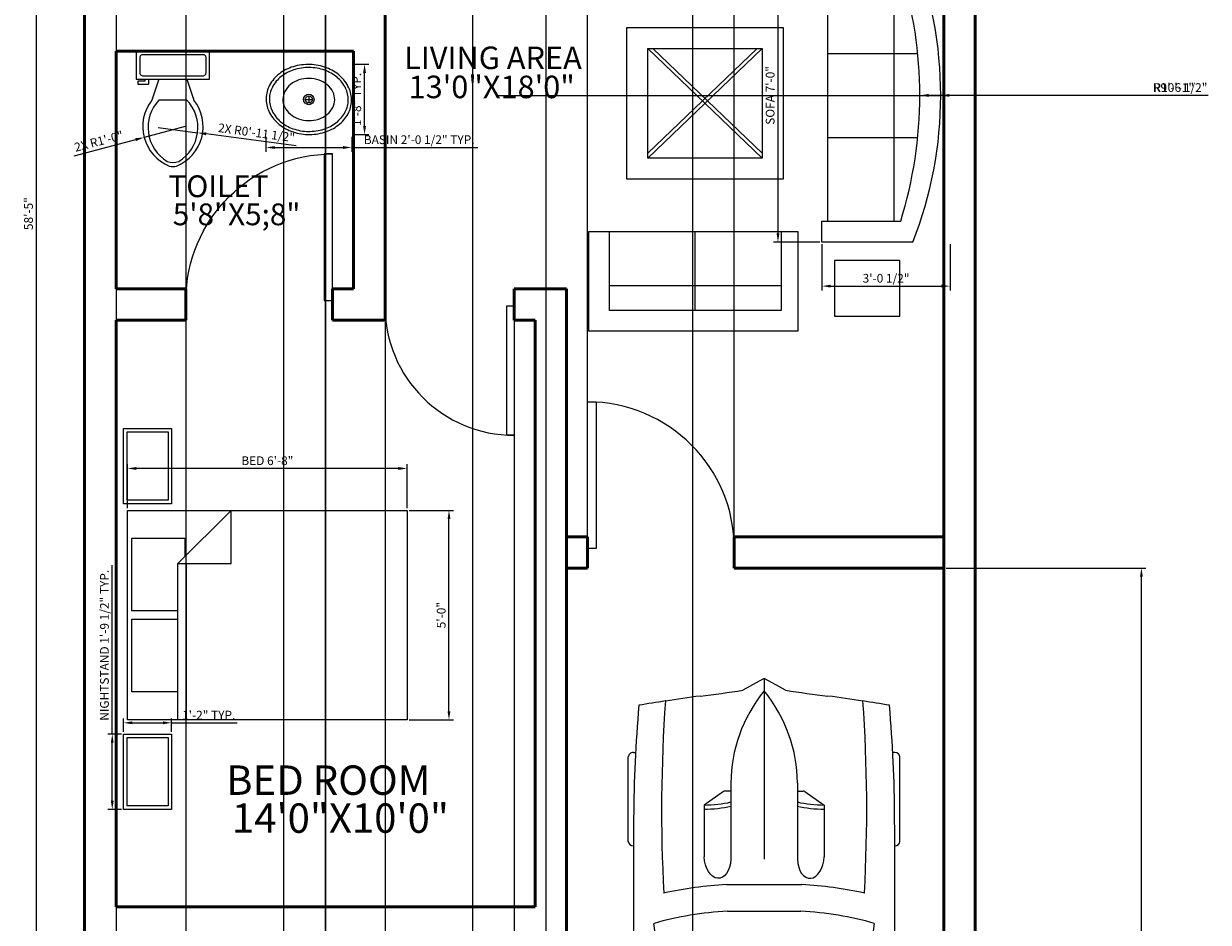
# Model space of a CAD drawing. Units: inches. Extents: x 758743 to 759108, y 3712801 to 3713581.
# Tile 2 of 4: x 758768 to 759108, y 3712987 to 3713244. Entities that reach past the tile are written whole.
import ezdxf

# ---------------------------------------------------------------- set-up
doc = ezdxf.new("R2010")
doc.units = ezdxf.units.IN
for name, color, linetype, lineweight in [('A-ANNO-DIMS', 2, 'Continuous', 18), ('A-AREA-IDEN', 3, 'Continuous', 18), ('A-FLOR-FIXT', 2, 'Continuous', 18), ('A-FURN', 2, 'Continuous', 18), ('A-SITE-VEHI', 8, 'Continuous', 13), ('DOOR', 4, 'Continuous', 25), ('WALL', 7, 'Continuous', 50)]:
    doc.layers.add(name, color=color, linetype=linetype, lineweight=lineweight)
doc.styles.get("Standard").update_dxf_attribs({"font": 'arial.ttf'})
doc.dimstyles.new('ISO-25', dxfattribs={"dimtxt": 2.5, "dimasz": 2.5, "dimexe": 1.25, "dimexo": 0.625, "dimtad": 1, "dimdec": 0, "dimlunit": 3, "dimtxsty": 'Standard', "dimcen": 2.5, "dimadec": 0, "dimazin": 0, "dimtfac": 1, "dimtdec": 0, "dimtmove": 0, "dimatfit": 3, "dimfxl": 1, "dimarcsym": 0})

# ---------------------------------------------------------------- blocks, each defined once
blk = doc.blocks.new('*U2')
for p, q in [((0, 0), (0, -100)), ((750, 0), (750, -100))]:
    blk.add_line(p, q)
blk.add_lwpolyline([(0, 0), (0, 750), (43.75, 750), (43.75, 0)], close=True)
blk.add_arc((0, 0), 750, 0, 90)
blk = doc.blocks.new('*U10')
for p, q in [((21.1, 37.41), (21.1, 36.83)), ((46.55, 38.89), (22.35, 38.89)), ((47.8, 37.39), (47.8, 37.41)), ((135.45, 37.07), (135.45, 37.41)), ((136.7, 38.89), (160.9, 38.89)), ((162.15, 37.41), (162.15, 36.77)), ((87.99, 31.87), (74.76, 35.92)), ((134.31, 35.6), (119.29, 31.78)), ((70.03, 31.54), (86.41, 29.35)), ((186.47, -33.5), (186.47, 33.5)), ((188.4, -32.76), (188.4, 32.76)), ((138.42, 29.35), (157.25, 29.35)), ((186.47, 29.35), (167.01, 29.35)), ((164.52, 26.39), (164.52, -26.39)), ((32.27, 11.63), (36.13, 17.17)), ((36.13, 17.17), (50.94, 17.17)), ((32.12, 9.51), (32.12, 11.15)), ((58.92, -10.77), (58.92, 10.77)), ((66.55, -10.53), (66.55, 10.53)), ((186.47, -10.53), (186.47, 10.53)), ((29.77, 9.51), (51.68, 9.51)), ((82.74, 8.5), (82.74, -8.5)), ((3.27, 6.13), (0.1, 0.41)), ((0, 0), (51.68, 0)), ((0.1, -0.41), (3.27, -6.13)), ((29.77, -9.51), (51.68, -9.51)), ((32.12, -9.51), (32.12, -11.15)), ((32.27, -11.63), (36.13, -17.17)), ((36.13, -17.17), (50.94, -17.17)), ((86.41, -29.35), (70.03, -31.54)), ((157.25, -29.35), (138.42, -29.35)), ((167.01, -29.35), (186.47, -29.35)), ((87.99, -31.87), (74.76, -35.92)), ((134.31, -35.6), (119.29, -31.78)), ((21.1, -37.41), (21.1, -36.83)), ((135.45, -37.07), (135.45, -37.41)), ((162.15, -37.41), (162.15, -36.77)), ((46.55, -38.89), (22.35, -38.89)), ((47.8, -37.39), (47.8, -37.41)), ((136.7, -38.89), (160.9, -38.89))]:
    blk.add_line(p, q)
for centre, major_axis, ratio, start_param, end_param in [((41.19, -490.86), (0, 528.23), 0.842304, 0.00281, 0.075598), ((22.35, 37.41), (0, -1.48), 0.842304, 3.141593, 4.712389), ((64.48, -10555.62), (0, 10593.03), 0.842304, -0.013397, 0.002797), ((46.55, 37.41), (0, 1.48), 0.842304, -1.570796, 0), ((136.7, 37.41), (0, -1.48), 0.842304, 3.141593, 4.712389), ((160.9, 37.41), (0, 1.48), 0.842304, -1.570796, 0), ((180.63, 35.84), (0, 2.22), 0.842304, -0.013017, 1.249894), ((64.48, -10556.36), (0, 10595.31), 0.842304, -0.013397, -0.013017), ((183.98, 32.76), (0, -5.25), 0.842304, 1.570796, 3.128196), ((266.03, -27.52), (0, 313.31), 0.842304, 1.367076, 1.39176), ((64.48, -10555.62), (0, -10591.55), 0.842304, 3.133765, 3.140441), ((183.98, 33.5), (0, -2.96), 0.842304, 1.570796, 3.128196), ((135.29, 5.39), (0, 81.77), 0.842304, 1.245306, 1.50788), ((95.79, -3666.35), (0, -3698.24), 0.842304, 3.134049, 3.144098), ((259.18, -27.52), (0, -305.3), 0.842304, 4.528606, 4.561838), ((37.47, -593.96), (0, -623.33), 0.842304, 3.096046, 3.200911), ((134.4, 5.39), (0, -89.78), 0.842304, 4.449482, 4.652344), ((149.6, 2.8), (0, -79.58), 0.842304, 4.372215, 4.640744), ((17.08, 0), (0, 147.02), 0.842304, 4.511394, 4.913384), ((35.91, 0), (0, 147.02), 0.842304, 4.511394, 4.913384), ((167.01, 26.39), (0, 2.96), 0.842304, 0, 1.570796), ((-204.49, 52.4), (0, -250.96), 0.842304, 1.385369, 1.434372), ((13.04, 17.01), (0, 27.42), 0.842304, 4.435146, 4.718221), ((14.2, 17.01), (0, 27.42), 0.842304, 4.435146, 4.718221), ((50.79, 13.34), (6.34, -0.36), 0.603834, -1.395552, 1.581315), ((32.75, 11.15), (0, 0.74), 0.842304, 0.879714, 1.570796), ((29.77, -46.66), (0, 56.17), 0.842304, 0, 0.590319), ((0.62, 0), (0, -0.74), 0.842304, 4.131459, 5.293319), ((29.77, 46.66), (0, 56.17), 0.842304, 2.551274, 3.141593), ((-204.49, -52.4), (0, 250.96), 0.842304, -1.434372, -1.385369), ((13.04, -17.01), (0, -27.42), 0.842304, 1.564964, 1.848039), ((14.2, -17.01), (0, -27.42), 0.842304, 1.564964, 1.848039), ((149.6, -2.8), (0, -79.58), 0.842304, -1.499151, -1.230623), ((32.75, -11.15), (0, -0.74), 0.842304, 4.712389, 5.403472), ((134.4, -5.39), (0, -89.78), 0.842304, -1.510751, -1.307889), ((135.29, -5.39), (0, -81.77), 0.842304, -1.50788, -1.245306), ((259.18, 27.52), (0, 305.3), 0.842304, 1.721348, 1.754579), ((167.01, -26.39), (0, -2.96), 0.842304, 4.712389, 6.283185), ((266.03, 27.52), (0, 313.31), 0.842304, 1.749832, 1.774517), ((37.47, 593.96), (0, -623.33), 0.842304, -0.059319, 0.045547), ((95.79, 3666.35), (0, -3698.24), 0.842304, -0.002505, 0.007544), ((183.98, -33.5), (0, 2.96), 0.842304, 3.15499, 4.712389), ((183.98, -32.76), (0, -5.25), 0.842304, 0.013397, 1.570796), ((41.19, 490.86), (0, -528.23), 0.842304, -0.075598, -0.00281), ((64.48, 10555.62), (0, 10593.03), 0.842304, 3.138796, 3.15499), ((64.48, 10555.62), (0, -10591.55), 0.842304, 0.001152, 0.007828), ((180.63, -35.84), (0, -2.22), 0.842304, -1.249894, 0.013017), ((22.35, -37.41), (0, 1.48), 0.842304, 1.570796, 3.141593), ((46.55, -37.41), (0, -1.48), 0.842304, 0, 1.570796), ((136.7, -37.41), (0, -1.48), 0.842304, -1.570796, 0), ((160.9, -37.41), (0, 1.48), 0.842304, 3.141593, 4.712389), ((64.48, 10556.36), (0, 10595.31), 0.842304, 3.15461, 3.15499)]:
    blk.add_ellipse(centre, major_axis=major_axis, ratio=ratio, start_param=start_param, end_param=end_param)
at = {"extrusion": (0, 0, -1)}
blk.add_ellipse((50.79, -13.34), major_axis=(6.34, 0.36), ratio=0.603834, start_param=-1.395552, end_param=1.581315, dxfattribs=at)
blk = doc.blocks.new('Toilet - top')
for p, q in [((9.5, -6), (9.5, -2)), ((-10, -8.5), (-8, -8.5)), ((-10, -9.5), (-10, -8.5)), ((-7, -9.5), (-10, -9.5)), ((-8, -8.5), (-8, -8)), ((-7, -8), (-7, -9.5)), ((-4, -8), (-6, -14)), ((4, -8), (6, -14)), ((4, -14), (-4, -14))]:
    blk.add_line(p, q)
blk.add_lwpolyline([(10.5, -8), (10.5, 0), (-10.5, 0), (-10.5, -8)], close=True)
for points in [[(-9.5, -2), (-9.5, -6)], [(8.5, -1), (-8.5, -1)], [(-8.5, -7), (8.5, -7)]]:
    blk.add_lwpolyline(points)
for centre, radius, start, end in [((-8.62, -1.88), 0.884, 81.8699, 188.1301), ((8.62, -1.88), 0.884, 351.8699, 98.1301), ((-8.62, -6.12), 0.884, 171.8699, 278.1301), ((8.62, -6.12), 0.884, 261.8699, 8.1301), ((3.52, -21.58), 12.17, 141.4691, 247.9714), ((4.2, -21.82), 11.33, 136.3677, 238.9468), ((-3.52, -21.58), 12.17, 292.0284, 38.5307), ((-4.2, -21.82), 11.33, 301.053, 43.6321), ((0, -27.88), 4, 245.7318, 294.2682), ((0, -29), 4, 254.8605, 285.1395)]:
    blk.add_arc(centre, radius, start, end)
blk = doc.blocks.new('Bed - Queen')
for p, q in [((0, -80.00003), (0, 0)), ((0, 0), (59.99999, 0)), ((59.99999, 0), (59.99999, -80.00003)), ((7.99999, -1.2), (28.79998, -1.2)), ((7.99999, -14.4), (7.99999, -1.2)), ((28.79998, -1.2), (28.79998, -14.4)), ((31.19999, -1.2), (51.99999, -1.2)), ((31.19999, -14.4), (31.19999, -1.2)), ((51.99999, -1.2), (51.99999, -16.4)), ((0, -14.4), (44.8, -14.4)), ((44.8, -16.8), (0, -16.8)), ((59.99999, -29.6), (44.8, -14.4)), ((44.8, -14.4), (44.8, -29.6)), ((51.99999, -16.4), (46.79936, -16.4)), ((44.8, -29.6), (59.99999, -29.6)), ((59.99999, -80.00003), (0, -80.00003))]:
    blk.add_line(p, q)
blk = doc.blocks.new('Sink - Oval top')
for p, q in [((-1, 0), (1, 0)), ((0, 1), (0, -1))]:
    blk.add_line(p, q)
for points in [[(-12.23, 0.39, 0.117634), (-11.46, -3.36, 0.104469), (-8.88, -6.8, 0.090016), (-5.08, -9.07, 0.08192), (-0.32, -10.02, 0.08192), (4.49, -9.38, 0.090016), (8.42, -7.36, 0.104469), (11.22, -4.09, 0.117634), (12.23, -0.39, 0.117634), (11.46, 3.36, 0.104469), (8.88, 6.8, 0.090016), (5.08, 9.07, 0.08192), (0.32, 10.02, 0.08192), (-4.49, 9.38, 0.090016), (-8.42, 7.36, 0.104469), (-11.22, 4.09, 0.117634)], [(-11.29, 0.16, 0.118622), (-10.52, -3.25, 0.104678), (-8.07, -6.36, 0.089562), (-4.54, -8.37, 0.081185), (-0.13, -9.15, 0.081185), (4.3, -8.49, 0.089562), (7.89, -6.58, 0.104678), (10.42, -3.55, 0.118622), (11.29, -0.16, 0.118622), (10.52, 3.25, 0.104678), (8.07, 6.36, 0.089562), (4.54, 8.37, 0.081185), (0.13, 9.15, 0.081185), (-4.3, 8.49, 0.089562), (-7.89, 6.58, 0.104678), (-10.42, 3.55, 0.118622)], [(-7.42, 0.08, 0.118283), (-6.91, -2.17, 0.104607), (-5.29, -4.21, 0.089718), (-2.97, -5.53, 0.081436), (-0.07, -6.04, 0.081436), (2.84, -5.59, 0.089718), (5.2, -4.33, 0.104607), (6.86, -2.32, 0.118283), (7.42, -0.08, 0.118283), (6.91, 2.17, 0.104607), (5.29, 4.21, 0.089718), (2.97, 5.53, 0.081436), (0.07, 6.04, 0.081436), (-2.84, 5.59, 0.089718), (-5.2, 4.33, 0.104607), (-6.86, 2.32, 0.118283)]]:
    blk.add_lwpolyline(points, format="xyb", close=True)
for radius in [1.5, 1]:
    blk.add_circle((0, 0), radius)
blk = doc.blocks.new('Sofa - Roundback 7 ft.')
for p, q in [((-12.00002, -32.4421), (-12.00003, -6.5971)), ((11.99997, -32.4421), (11.99998, -6.5971)), ((-36.000027, -34), (-36.000027, -11.4696)), ((-35.999844, -13.3819), (35.9998, -13.3819)), ((35.99998, -34), (35.99998, -11.4696)), ((-36.000027, -32.4421), (35.99998, -32.4421))]:
    blk.add_line(p, q)
for points in [[(-36.000027, -34), (-42.000027, -34), (-42.000027, -8)], [(41.99998, -8), (41.99998, -34), (35.99998, -34)]]:
    blk.add_lwpolyline(points)
for centre, radius, start, end in [((0, -114.25), 114.25, 68.43141, 111.5686), ((-0.00001, -127.1968), 121.1968, 72.72033, 107.2797)]:
    blk.add_arc(centre, radius, start, end)
blk = doc.blocks.new('*D13')
at = {"layer": 'A-ANNO-DIMS', "color": 0, "lineweight": -2, "transparency": 16777216}
for p, q in [((758785.26, 3713540.49), (758770.79, 3713540.49)), ((758772.04, 3713537.99), (758772.04, 3712841.99)), ((758785.26, 3712839.49), (758770.79, 3712839.49))]:
    blk.add_line(p, q, dxfattribs=at)
at = {"layer": 'A-ANNO-DIMS', "color": 0, "transparency": 16777216}
for points in [[(758771.62, 3713537.99), (758772.46, 3713537.99), (758772.04, 3713540.49)], [(758771.62, 3712841.99), (758772.46, 3712841.99), (758772.04, 3712839.49)]]:
    blk.add_solid(points, dxfattribs=at)
at = {"layer": 'Defpoints', "color": 0, "transparency": 16777216}
for p in [(758785.89, 3713540.49), (758772.04, 3712839.49), (758785.89, 3712839.49)]:
    blk.add_point(p, dxfattribs=at)
at = {"layer": 'A-ANNO-DIMS', "color": 0, "transparency": 16777216, "insert": (758770.14, 3713189.99), "char_height": 2.5, "attachment_point": 5, "rotation": 90}
blk.add_mtext('58\'-5"', dxfattribs=at)
blk = doc.blocks.new('NIGHTSTAND-LARGE')
for points in [[(0, 21.57), (13.76, 21.57), (13.76, 0), (0, 0)], [(1, 20.57), (12.76, 20.57), (12.76, 1), (1, 1)]]:
    blk.add_lwpolyline(points, close=True)
blk = doc.blocks.new('END-TABLE')
blk.add_lwpolyline([(0, 15.93), (18.69, 15.93), (18.69, 0), (0, 0)], close=True)
blk = doc.blocks.new('*D24')
at = {"layer": 'A-ANNO-DIMS', "color": 0, "lineweight": -2, "transparency": 16777216}
for p, q in [((758837.79, 3713211.98), (758837.79, 3713207.68)), ((758862.34, 3713211.98), (758862.34, 3713207.68)), ((758840.29, 3713208.93), (758859.84, 3713208.93)), ((758862.34, 3713208.93), (758898.5, 3713208.93))]:
    blk.add_line(p, q, dxfattribs=at)
at = {"layer": 'A-ANNO-DIMS', "color": 0, "transparency": 16777216}
for points in [[(758840.29, 3713209.34), (758840.29, 3713208.51), (758837.79, 3713208.93)], [(758859.84, 3713209.34), (758859.84, 3713208.51), (758862.34, 3713208.93)]]:
    blk.add_solid(points, dxfattribs=at)
at = {"layer": 'Defpoints', "color": 0, "transparency": 16777216}
for p in [(758837.79, 3713212.61), (758862.34, 3713212.61), (758862.34, 3713208.93)]:
    blk.add_point(p, dxfattribs=at)
at = {"layer": 'A-ANNO-DIMS', "color": 0, "transparency": 16777216, "insert": (758881.67, 3713210.84), "char_height": 2.5, "attachment_point": 5}
blk.add_mtext('BASIN 2\'-0 1/2" TYP.', dxfattribs=at)
blk = doc.blocks.new('*D25')
at = {"layer": 'A-ANNO-DIMS', "color": 0, "lineweight": -2, "transparency": 16777216}
for p, q in [((758862.97, 3713232.75), (758867.27, 3713232.75)), ((758866.02, 3713215.11), (758866.02, 3713230.25)), ((758862.97, 3713212.61), (758867.27, 3713212.61))]:
    blk.add_line(p, q, dxfattribs=at)
at = {"layer": 'A-ANNO-DIMS', "color": 0, "transparency": 16777216}
for points in [[(758865.61, 3713230.25), (758866.44, 3713230.25), (758866.02, 3713232.75)], [(758865.61, 3713215.11), (758866.44, 3713215.11), (758866.02, 3713212.61)]]:
    blk.add_solid(points, dxfattribs=at)
at = {"layer": 'Defpoints', "color": 0, "transparency": 16777216}
for p in [(758862.34, 3713232.75), (758866.02, 3713232.75), (758862.34, 3713212.61)]:
    blk.add_point(p, dxfattribs=at)
at = {"layer": 'A-ANNO-DIMS', "color": 0, "transparency": 16777216, "insert": (758864.12, 3713222.68), "char_height": 2.5, "attachment_point": 5, "rotation": 90}
blk.add_mtext('1\'-8" TYP.', dxfattribs=at)
blk = doc.blocks.new('*D26')
at = {"layer": 'A-ANNO-DIMS', "color": 0, "lineweight": -2, "transparency": 16777216}
for p, q in [((758798.2, 3713105.65), (758798.2, 3713118.27)), ((758875.7, 3713117.02), (758800.7, 3713117.02)), ((758878.2, 3713105.65), (758878.2, 3713118.27))]:
    blk.add_line(p, q, dxfattribs=at)
at = {"layer": 'A-ANNO-DIMS', "color": 0, "transparency": 16777216}
for points in [[(758800.7, 3713117.44), (758800.7, 3713116.6), (758798.2, 3713117.02)], [(758875.7, 3713117.44), (758875.7, 3713116.6), (758878.2, 3713117.02)]]:
    blk.add_solid(points, dxfattribs=at)
at = {"layer": 'Defpoints', "color": 0, "transparency": 16777216}
for p in [(758798.2, 3713117.02), (758798.2, 3713105.02), (758878.2, 3713105.02)]:
    blk.add_point(p, dxfattribs=at)
at = {"layer": 'A-ANNO-DIMS', "color": 0, "transparency": 16777216, "insert": (758838.2, 3713118.92), "char_height": 2.5, "attachment_point": 5}
blk.add_mtext('BED 6\'-8"', dxfattribs=at)
blk = doc.blocks.new('*D27')
at = {"layer": 'A-ANNO-DIMS', "color": 0, "lineweight": -2, "transparency": 16777216}
for p, q in [((758878.83, 3713105.02), (758891.45, 3713105.02)), ((758890.2, 3713047.52), (758890.2, 3713102.52)), ((758878.83, 3713045.02), (758891.45, 3713045.02))]:
    blk.add_line(p, q, dxfattribs=at)
at = {"layer": 'A-ANNO-DIMS', "color": 0, "transparency": 16777216}
for points in [[(758889.78, 3713102.52), (758890.62, 3713102.52), (758890.2, 3713105.02)], [(758889.78, 3713047.52), (758890.62, 3713047.52), (758890.2, 3713045.02)]]:
    blk.add_solid(points, dxfattribs=at)
at = {"layer": 'Defpoints', "color": 0, "transparency": 16777216}
for p in [(758878.2, 3713105.02), (758890.2, 3713105.02), (758878.2, 3713045.02)]:
    blk.add_point(p, dxfattribs=at)
at = {"layer": 'A-ANNO-DIMS', "color": 0, "transparency": 16777216, "insert": (758888.3, 3713075.02), "char_height": 2.5, "attachment_point": 5, "rotation": 90}
blk.add_mtext('5\'-0"', dxfattribs=at)
blk = doc.blocks.new('*D30')
at = {"layer": 'A-ANNO-DIMS', "color": 0, "lineweight": -2, "transparency": 16777216}
for p, q in [((758793.79, 3713040.96), (758793.79, 3713089.32)), ((758796.4, 3713040.96), (758792.54, 3713040.96)), ((758793.79, 3713021.89), (758793.79, 3713038.46)), ((758796.4, 3713019.39), (758792.54, 3713019.39))]:
    blk.add_line(p, q, dxfattribs=at)
at = {"layer": 'A-ANNO-DIMS', "color": 0, "transparency": 16777216}
for points in [[(758793.37, 3713038.46), (758794.21, 3713038.46), (758793.79, 3713040.96)], [(758793.37, 3713021.89), (758794.21, 3713021.89), (758793.79, 3713019.39)]]:
    blk.add_solid(points, dxfattribs=at)
at = {"layer": 'Defpoints', "color": 0, "transparency": 16777216}
for p in [(758793.79, 3713040.96), (758797.02, 3713040.96), (758797.02, 3713019.39)]:
    blk.add_point(p, dxfattribs=at)
at = {"layer": 'A-ANNO-DIMS', "color": 0, "transparency": 16777216, "insert": (758791.87, 3713066.39), "char_height": 2.5, "attachment_point": 5, "rotation": 90}
blk.add_mtext('NIGHTSTAND 1\'-9 1/2" TYP.', dxfattribs=at)
blk = doc.blocks.new('*D31')
at = {"layer": 'A-ANNO-DIMS', "color": 0, "lineweight": -2, "transparency": 16777216}
for p, q in [((758797.02, 3713041.58), (758797.02, 3713045.44)), ((758799.52, 3713044.19), (758808.28, 3713044.19)), ((758810.78, 3713041.58), (758810.78, 3713045.44)), ((758810.78, 3713044.19), (758829.54, 3713044.19))]:
    blk.add_line(p, q, dxfattribs=at)
at = {"layer": 'A-ANNO-DIMS', "color": 0, "transparency": 16777216}
for points in [[(758799.52, 3713044.61), (758799.52, 3713043.78), (758797.02, 3713044.19)], [(758808.28, 3713044.61), (758808.28, 3713043.78), (758810.78, 3713044.19)]]:
    blk.add_solid(points, dxfattribs=at)
at = {"layer": 'Defpoints', "color": 0, "transparency": 16777216}
for p in [(758810.78, 3713044.19), (758797.02, 3713040.96), (758810.78, 3713040.96)]:
    blk.add_point(p, dxfattribs=at)
at = {"layer": 'A-ANNO-DIMS', "color": 0, "transparency": 16777216, "insert": (758821.41, 3713046.07), "char_height": 2.5, "attachment_point": 5}
blk.add_mtext('1\'-2" TYP.', dxfattribs=at)
blk = doc.blocks.new('*D40')
at = {"layer": 'A-ANNO-DIMS', "color": 0, "lineweight": -2, "transparency": 16777216}
for p, q in [((758996.38, 3713265.84), (758983.15, 3713265.84)), ((758984.4, 3713263.34), (758984.4, 3713184.34)), ((758996.38, 3713181.84), (758983.15, 3713181.84))]:
    blk.add_line(p, q, dxfattribs=at)
at = {"layer": 'A-ANNO-DIMS', "color": 0, "transparency": 16777216}
for points in [[(758983.99, 3713263.34), (758984.82, 3713263.34), (758984.4, 3713265.84)], [(758983.99, 3713184.34), (758984.82, 3713184.34), (758984.4, 3713181.84)]]:
    blk.add_solid(points, dxfattribs=at)
at = {"layer": 'Defpoints', "color": 0, "transparency": 16777216}
for p in [(758997, 3713265.84), (758984.4, 3713181.84), (758997, 3713181.84)]:
    blk.add_point(p, dxfattribs=at)
at = {"layer": 'A-ANNO-DIMS', "color": 0, "transparency": 16777216, "insert": (758982.48, 3713223.84), "char_height": 2.5, "attachment_point": 5, "rotation": 90}
blk.add_mtext('SOFA 7\'-0"', dxfattribs=at)
blk = doc.blocks.new('*D41')
at = {"layer": 'A-ANNO-DIMS', "color": 0, "lineweight": -2, "transparency": 16777216}
for p, q in [((758997, 3713181.22), (758997, 3713167.99)), ((759033.67, 3713181.22), (759033.67, 3713167.99)), ((758999.5, 3713169.24), (759031.17, 3713169.24))]:
    blk.add_line(p, q, dxfattribs=at)
at = {"layer": 'A-ANNO-DIMS', "color": 0, "transparency": 16777216}
for points in [[(758999.5, 3713169.66), (758999.5, 3713168.83), (758997, 3713169.24)], [(759031.17, 3713169.66), (759031.17, 3713168.83), (759033.67, 3713169.24)]]:
    blk.add_solid(points, dxfattribs=at)
at = {"layer": 'Defpoints', "color": 0, "transparency": 16777216}
for p in [(758997, 3713181.84), (759033.67, 3713181.84), (759033.67, 3713169.24)]:
    blk.add_point(p, dxfattribs=at)
at = {"layer": 'A-ANNO-DIMS', "color": 0, "transparency": 16777216, "insert": (759015.34, 3713171.16), "char_height": 2.5, "attachment_point": 5}
blk.add_mtext('3\'-0 1/2"', dxfattribs=at)
blk = doc.blocks.new('*D46')
at = {"layer": 'A-ANNO-DIMS', "color": 0, "lineweight": -2, "transparency": 16777216}
for p, q in [((758842.89, 3712849.12), (758842.89, 3713578.64)), ((758854.89, 3712849.12), (758854.89, 3713578.64)), ((758845.39, 3713577.39), (758852.39, 3713577.39))]:
    blk.add_line(p, q, dxfattribs=at)
at = {"layer": 'A-ANNO-DIMS', "color": 0, "transparency": 16777216}
for points in [[(758845.39, 3713577.81), (758845.39, 3713576.97), (758842.89, 3713577.39)], [(758852.39, 3713577.81), (758852.39, 3713576.97), (758854.89, 3713577.39)]]:
    blk.add_solid(points, dxfattribs=at)
at = {"layer": 'Defpoints', "color": 0, "transparency": 16777216}
for p in [(758854.89, 3713577.39), (758842.89, 3712848.49), (758854.89, 3712848.49)]:
    blk.add_point(p, dxfattribs=at)
at = {"layer": 'A-ANNO-DIMS', "color": 0, "transparency": 16777216, "insert": (758848.89, 3713579.29), "char_height": 2.5, "attachment_point": 5}
blk.add_mtext('1\'-0"', dxfattribs=at)
blk = doc.blocks.new('*D49')
at = {"layer": 'A-ANNO-DIMS', "color": 0, "lineweight": -2, "transparency": 16777216}
for p, q in [((758929.89, 3713089.12), (758929.89, 3713578.64)), ((758971.89, 3713089.12), (758971.89, 3713578.64)), ((758932.39, 3713577.39), (758969.39, 3713577.39))]:
    blk.add_line(p, q, dxfattribs=at)
at = {"layer": 'A-ANNO-DIMS', "color": 0, "transparency": 16777216}
for points in [[(758932.39, 3713577.81), (758932.39, 3713576.97), (758929.89, 3713577.39)], [(758969.39, 3713577.81), (758969.39, 3713576.97), (758971.89, 3713577.39)]]:
    blk.add_solid(points, dxfattribs=at)
at = {"layer": 'Defpoints', "color": 0, "transparency": 16777216}
for p in [(758971.89, 3713577.39), (758929.89, 3713088.49), (758971.89, 3713088.49)]:
    blk.add_point(p, dxfattribs=at)
at = {"layer": 'A-ANNO-DIMS', "color": 0, "transparency": 16777216, "insert": (758950.89, 3713579.29), "char_height": 2.5, "attachment_point": 5}
blk.add_mtext('3\'-6"', dxfattribs=at)
blk = doc.blocks.new('*D50')
at = {"layer": 'A-ANNO-DIMS', "color": 0, "lineweight": -2, "transparency": 16777216}
for p, q in [((758794.89, 3713312.87), (758794.89, 3712801.34)), ((758814.89, 3713312.87), (758814.89, 3712801.34)), ((758797.39, 3712802.59), (758812.39, 3712802.59))]:
    blk.add_line(p, q, dxfattribs=at)
at = {"layer": 'A-ANNO-DIMS', "color": 0, "transparency": 16777216}
for points in [[(758797.39, 3712803.01), (758797.39, 3712802.17), (758794.89, 3712802.59)], [(758812.39, 3712803.01), (758812.39, 3712802.17), (758814.89, 3712802.59)]]:
    blk.add_solid(points, dxfattribs=at)
at = {"layer": 'Defpoints', "color": 0, "transparency": 16777216}
for p in [(758794.89, 3713313.49), (758814.89, 3713313.49), (758814.89, 3712802.59)]:
    blk.add_point(p, dxfattribs=at)
at = {"layer": 'A-ANNO-DIMS', "color": 0, "transparency": 16777216, "insert": (758804.89, 3712804.49), "char_height": 2.5, "attachment_point": 5}
blk.add_mtext('1\'-8"', dxfattribs=at)
blk = doc.blocks.new('*D52')
at = {"layer": 'A-ANNO-DIMS', "color": 0, "lineweight": -2, "transparency": 16777216}
for p, q in [((758871.89, 3713158.87), (758871.89, 3712801.34)), ((758908.89, 3713158.87), (758908.89, 3712801.34)), ((758874.39, 3712802.59), (758906.39, 3712802.59))]:
    blk.add_line(p, q, dxfattribs=at)
at = {"layer": 'A-ANNO-DIMS', "color": 0, "transparency": 16777216}
for points in [[(758874.39, 3712803.01), (758874.39, 3712802.17), (758871.89, 3712802.59)], [(758906.39, 3712803.01), (758906.39, 3712802.17), (758908.89, 3712802.59)]]:
    blk.add_solid(points, dxfattribs=at)
at = {"layer": 'Defpoints', "color": 0, "transparency": 16777216}
for p in [(758871.89, 3713159.49), (758908.89, 3713159.49), (758908.89, 3712802.59)]:
    blk.add_point(p, dxfattribs=at)
at = {"layer": 'A-ANNO-DIMS', "color": 0, "transparency": 16777216, "insert": (758890.39, 3712804.49), "char_height": 2.5, "attachment_point": 5}
blk.add_mtext('3\'-1"', dxfattribs=at)
blk = doc.blocks.new('*D54')
at = {"layer": 'A-ANNO-DIMS', "color": 0, "lineweight": -2, "transparency": 16777216}
for p, q in [((758854.89, 3713405.87), (758854.89, 3712801.34)), ((758896.89, 3713405.87), (758896.89, 3712801.34)), ((758857.39, 3712802.59), (758894.39, 3712802.59))]:
    blk.add_line(p, q, dxfattribs=at)
at = {"layer": 'A-ANNO-DIMS', "color": 0, "transparency": 16777216}
for points in [[(758857.39, 3712803.01), (758857.39, 3712802.17), (758854.89, 3712802.59)], [(758894.39, 3712803.01), (758894.39, 3712802.17), (758896.89, 3712802.59)]]:
    blk.add_solid(points, dxfattribs=at)
at = {"layer": 'Defpoints', "color": 0, "transparency": 16777216}
for p in [(758854.89, 3713406.49), (758896.89, 3713406.49), (758896.89, 3712802.59)]:
    blk.add_point(p, dxfattribs=at)
at = {"layer": 'A-ANNO-DIMS', "color": 0, "transparency": 16777216, "insert": (758875.89, 3712804.49), "char_height": 2.5, "attachment_point": 5}
blk.add_mtext('3\'-6"', dxfattribs=at)
blk = doc.blocks.new('*D55')
at = {"layer": 'A-ANNO-DIMS', "color": 0, "lineweight": -2, "transparency": 16777216}
for p, q in [((759032.51, 3713088.49), (759089.7, 3713088.49)), ((759088.45, 3712850.99), (759088.45, 3713085.99)), ((759032.51, 3712848.49), (759089.7, 3712848.49))]:
    blk.add_line(p, q, dxfattribs=at)
at = {"layer": 'A-ANNO-DIMS', "color": 0, "transparency": 16777216}
for points in [[(759088.04, 3713085.99), (759088.87, 3713085.99), (759088.45, 3713088.49)], [(759088.04, 3712850.99), (759088.87, 3712850.99), (759088.45, 3712848.49)]]:
    blk.add_solid(points, dxfattribs=at)
at = {"layer": 'Defpoints', "color": 0, "transparency": 16777216}
for p in [(759031.89, 3713088.49), (759088.45, 3713088.49), (759031.89, 3712848.49)]:
    blk.add_point(p, dxfattribs=at)
at = {"layer": 'A-ANNO-DIMS', "color": 0, "transparency": 16777216, "insert": (759086.55, 3712968.49), "char_height": 2.5, "attachment_point": 5, "rotation": 90}
blk.add_mtext('20\'-0"', dxfattribs=at)
blk = doc.blocks.new('*D59')
at = {"layer": 'A-ANNO-DIMS', "color": 0, "lineweight": -2, "transparency": 16777216}
for p, q in [((758917.89, 3713405.87), (758917.89, 3712801.34)), ((758959.89, 3713405.87), (758959.89, 3712801.34)), ((758920.39, 3712802.59), (758957.39, 3712802.59))]:
    blk.add_line(p, q, dxfattribs=at)
at = {"layer": 'A-ANNO-DIMS', "color": 0, "transparency": 16777216}
for points in [[(758920.39, 3712803.01), (758920.39, 3712802.17), (758917.89, 3712802.59)], [(758957.39, 3712803.01), (758957.39, 3712802.17), (758959.89, 3712802.59)]]:
    blk.add_solid(points, dxfattribs=at)
at = {"layer": 'Defpoints', "color": 0, "transparency": 16777216}
for p in [(758917.89, 3713406.49), (758959.89, 3713406.49), (758959.89, 3712802.59)]:
    blk.add_point(p, dxfattribs=at)
at = {"layer": 'A-ANNO-DIMS', "color": 0, "transparency": 16777216, "insert": (758938.89, 3712804.49), "char_height": 2.5, "attachment_point": 5}
blk.add_mtext('3\'-6"', dxfattribs=at)
blk = doc.blocks.new('*D61')
at = {"layer": 'A-ANNO-DIMS', "color": 0, "lineweight": -2, "transparency": 16777216}
for p, q in [((758903.81, 3713223.84), (759025, 3713223.84)), ((759103.84, 3713223.84), (759027.5, 3713223.84))]:
    blk.add_line(p, q, dxfattribs=at)
at = {"layer": 'A-ANNO-DIMS', "color": 0, "transparency": 16777216}
blk.add_solid([(759027.5, 3713224.26), (759027.5, 3713223.43), (759025, 3713223.84)], dxfattribs=at)
at = {"layer": 'Defpoints', "color": 0, "transparency": 16777216}
for p in [(758903.81, 3713223.84), (759025, 3713223.84)]:
    blk.add_point(p, dxfattribs=at)
at = {"layer": 'A-ANNO-DIMS', "color": 0, "transparency": 16777216, "insert": (759097.72, 3713225.75), "char_height": 2.5, "attachment_point": 5, "rotation": 0.0001}
blk.add_mtext('R10\'-1"', dxfattribs=at)
blk = doc.blocks.new('*D62')
at = {"layer": 'A-ANNO-DIMS', "color": 0, "lineweight": -2, "transparency": 16777216}
for p, q in [((758916.75, 3713223.84), (759031, 3713223.84)), ((759107.61, 3713223.84), (759033.5, 3713223.84))]:
    blk.add_line(p, q, dxfattribs=at)
at = {"layer": 'A-ANNO-DIMS', "color": 0, "transparency": 16777216}
blk.add_solid([(759033.5, 3713224.26), (759033.5, 3713223.43), (759031, 3713223.84)], dxfattribs=at)
at = {"layer": 'Defpoints', "color": 0, "transparency": 16777216}
for p in [(758916.75, 3713223.84), (759031, 3713223.84)]:
    blk.add_point(p, dxfattribs=at)
at = {"layer": 'A-ANNO-DIMS', "color": 0, "transparency": 16777216, "insert": (759099.55, 3713225.76), "char_height": 2.5, "attachment_point": 5, "rotation": 0.0001}
blk.add_mtext('R9\'-6 1/2"', dxfattribs=at)
blk = doc.blocks.new('*D65')
at = {"layer": 'A-ANNO-DIMS', "color": 0, "lineweight": -2, "transparency": 16777216}
for p, q in [((758814.69, 3713214.91), (758802.92, 3713211.82)), ((758782.9, 3713206.56), (758800.51, 3713211.18))]:
    blk.add_line(p, q, dxfattribs=at)
at = {"layer": 'A-ANNO-DIMS', "color": 0, "transparency": 16777216}
blk.add_solid([(758800.4, 3713211.59), (758800.61, 3713210.78), (758802.92, 3713211.82)], dxfattribs=at)
at = {"layer": 'Defpoints', "color": 0, "transparency": 16777216}
for p in [(758814.69, 3713214.91), (758802.92, 3713211.82)]:
    blk.add_point(p, dxfattribs=at)
at = {"layer": 'A-ANNO-DIMS', "color": 0, "transparency": 16777216, "insert": (758790.01, 3713210.39), "char_height": 2.5, "attachment_point": 5, "rotation": 14.7202}
blk.add_mtext('2X R1\'-0"', dxfattribs=at)
blk = doc.blocks.new('*D66')
at = {"layer": 'A-ANNO-DIMS', "color": 0, "lineweight": -2, "transparency": 16777216}
for p, q in [((758806.97, 3713214.67), (758818.2, 3713213.16)), ((758846.42, 3713209.37), (758820.68, 3713212.83))]:
    blk.add_line(p, q, dxfattribs=at)
at = {"layer": 'A-ANNO-DIMS', "color": 0, "transparency": 16777216}
blk.add_solid([(758820.74, 3713213.24), (758820.62, 3713212.42), (758818.2, 3713213.16)], dxfattribs=at)
at = {"layer": 'Defpoints', "color": 0, "transparency": 16777216}
for p in [(758806.97, 3713214.67), (758818.2, 3713213.16)]:
    blk.add_point(p, dxfattribs=at)
at = {"layer": 'A-ANNO-DIMS', "color": 0, "transparency": 16777216, "insert": (758835.04, 3713212.84), "char_height": 2.5, "attachment_point": 5, "rotation": 352.3445}
blk.add_mtext('2X R0\'-11 1/2"', dxfattribs=at)

msp = doc.modelspace()

# ---------------------------------------------------------------- linework, layer by layer
at = {"layer": 'A-FURN'}
for p, q in [((758947.17, 3713205.88), (758979.87, 3713237.27)), ((758979.87, 3713205.88), (758947.17, 3713237.27)), ((758947.17, 3713207.26), (758978.43, 3713237.27)), ((758979.87, 3713207.26), (758948.61, 3713237.27)), ((758936.13, 3713162.3), (758936.13, 3713184.86)), ((758960.72, 3713162.3), (758960.72, 3713184.86)), ((758985.3, 3713184.86), (758985.3, 3713162.3)), ((758936.13, 3713169.39), (758985.3, 3713169.39)), ((758985.3, 3713162.3), (758936.13, 3713162.3))]:
    msp.add_line(p, q, dxfattribs=at)
for points in [[(758941.17, 3713243.27), (758985.87, 3713243.27), (758985.87, 3713199.88), (758941.17, 3713199.88)], [(758947.17, 3713237.27), (758979.87, 3713237.27), (758979.87, 3713205.88), (758947.17, 3713205.88)], [(758930.25, 3713184.86), (758990.04, 3713184.86), (758990.04, 3713156.32), (758930.25, 3713156.32)]]:
    msp.add_lwpolyline(points, close=True, dxfattribs=at)
at = {"layer": 'WALL'}
for p, q in [((758785.89, 3713540.49), (758785.89, 3712839.49)), ((759040.89, 3713540.49), (759040.89, 3712839.49)), ((759031.89, 3713406.49), (759031.89, 3712848.49)), ((758871.89, 3713322.49), (758871.89, 3713159.49)), ((758794.89, 3713236.49), (758862.89, 3713236.49)), ((758794.89, 3713236.49), (758794.89, 3713168.49)), ((758862.89, 3713236.49), (758862.89, 3713168.49)), ((758794.89, 3713168.49), (758814.89, 3713168.49)), ((758794.89, 3713168.49), (758814.89, 3713168.49)), ((758814.89, 3713159.49), (758814.89, 3713168.49)), ((758856.89, 3713159.49), (758856.89, 3713168.49)), ((758856.89, 3713168.49), (758862.89, 3713168.49)), ((758856.89, 3713168.49), (758862.89, 3713168.49)), ((758908.89, 3713168.49), (758923.89, 3713168.49)), ((758908.89, 3713159.49), (758908.89, 3713168.49)), ((758923.89, 3713168.49), (758923.89, 3713097.49)), ((758794.89, 3713159.49), (758814.89, 3713159.49)), ((758794.89, 3713159.49), (758794.89, 3712991.49)), ((758856.89, 3713159.49), (758871.89, 3713159.49)), ((758908.89, 3713159.49), (758914.89, 3713159.49)), ((758914.89, 3713159.49), (758914.89, 3712991.49)), ((758923.89, 3713097.49), (758929.89, 3713097.49)), ((758923.89, 3713097.49), (758923.89, 3712982.49)), ((758929.89, 3713097.49), (758929.89, 3713088.49)), ((758971.89, 3713097.49), (758971.89, 3713088.49)), ((758971.89, 3713097.49), (759031.89, 3713097.49)), ((758923.89, 3713088.49), (758929.89, 3713088.49)), ((758971.89, 3713088.49), (759031.89, 3713088.49)), ((758794.89, 3712991.49), (758914.89, 3712991.49))]:
    msp.add_line(p, q, dxfattribs=at)

# ---------------------------------------------------------------- block references
at = {"layer": 'A-FLOR-FIXT'}
for name, p in [('Toilet - top', (758811.17, 3713236.49)), ('Sink - Oval top', (758850.07, 3713222.68))]:
    msp.add_blockref(name, p, dxfattribs=at)
at = {"layer": 'A-FURN'}
for name, p, rotation in [('Sofa - Roundback 7 ft.', (759031, 3713223.84), 270), ('Bed - Queen', (758798.2, 3713045.02), 90)]:
    msp.add_blockref(name, p, dxfattribs=dict(at, rotation=rotation))
at = {"layer": 'A-FURN', "extrusion": (0, 0, -1), "zscale": -1, "rotation": 180}
msp.add_blockref('END-TABLE', (-759000.62, 3713176.55), dxfattribs=at)
at = {"layer": 'A-FURN'}
for p in [(758797.03, 3713106.92), (758797.03, 3713019.39)]:
    msp.add_blockref('NIGHTSTAND-LARGE', p, dxfattribs=at)
at = {"layer": 'A-SITE-VEHI', "rotation": 270}
msp.add_blockref('*U10', (758980.44, 3713056.78), dxfattribs=at)
at = {"layer": 'DOOR', "yscale": 0.0559999999999739, "zscale": 0.0559999999999739}
for p, xscale in [((758856.89, 3713165.09), -0.0559999999999739), ((758929.89, 3713094.09), 0.0559999999999739)]:
    msp.add_blockref('*U2', p, dxfattribs=dict(at, xscale=xscale))
at = {"layer": 'DOOR', "xscale": 0.0493817936930376, "yscale": 0.0493817936930376, "zscale": 0.0493817936930376, "rotation": 180}
msp.add_blockref('*U2', (758908.89, 3713163.55), dxfattribs=at)

# ---------------------------------------------------------------- texts
at = {"layer": 'A-AREA-IDEN'}
for s, height, p in [('LIVING AREA', 6.4524, (758877.36, 3713231.38)), ('13\'0"X18\'0"', 6.4524, (758878.64, 3713223.05)), ('TOILET', 6.233, (758809.9, 3713194.71)), ('5\'8"X5;8"', 6.233, (758811.13, 3713186.67)), ('BED ROOM', 8.421, (758826.4, 3713023.56)), ('14\'0"X10\'0"', 8.4209, (758828.06, 3713012.69))]:
    msp.add_text(s, height=height, dxfattribs=at).set_placement(p)

# ---------------------------------------------------------------- dimensions: what is measured, and where the dimension line sits
at = {"layer": 'A-ANNO-DIMS'}
for base, p1, p2, picture, middle in [((758854.89, 3713577.39), (758842.89, 3712848.49), (758854.89, 3712848.49), '*D46', (758848.89, 3713579.29)), ((758971.89, 3713577.39), (758929.89, 3713088.49), (758971.89, 3713088.49), '*D49', (758950.89, 3713579.29)), ((758896.89, 3712802.59), (758854.89, 3713406.49), (758896.89, 3713406.49), '*D54', (758875.89, 3712804.49)), ((758959.89, 3712802.59), (758917.89, 3713406.49), (758959.89, 3713406.49), '*D59', (758938.89, 3712804.49)), ((758814.89, 3712802.59), (758794.89, 3713313.49), (758814.89, 3713313.49), '*D50', (758804.89, 3712804.49)), ((759033.67, 3713169.24), (758997, 3713181.84), (759033.67, 3713181.84), '*D41', (759015.34, 3713171.16)), ((758908.89, 3712802.59), (758871.89, 3713159.49), (758908.89, 3713159.49), '*D52', (758890.39, 3712804.49))]:
    dim = msp.add_linear_dim(base=base, p1=p1, p2=p2, dimstyle='ISO-25', override={"dimdec": 1, "dimlfac": 1, "dimrnd": 0, "dimzin": 1, "dimdsep": 46, "dimlunit": 4, "dimfrac": 2}, dxfattribs=at)
    dim.commit()
    dim.dimension.update_dxf_attribs({"geometry": picture, "text_midpoint": middle})
for base, p1, p2, override, picture, middle in [((758772.04, 3712839.49), (758785.89, 3713540.49), (758785.89, 3712839.49), {"dimclrd": 0, "dimclre": 0, "dimclrt": 0}, '*D13', (758770.14, 3713189.99)), ((758890.2, 3713105.02), (758878.2, 3713045.02), (758878.2, 3713105.02), {"dimdec": 1, "dimlfac": 1, "dimrnd": 0, "dimzin": 1, "dimdsep": 46, "dimlunit": 4, "dimfrac": 2}, '*D27', (758888.3, 3713075.02)), ((759088.45, 3713088.49), (759031.89, 3712848.49), (759031.89, 3713088.49), {"dimdec": 1, "dimlfac": 1, "dimrnd": 0, "dimzin": 1, "dimdsep": 46, "dimlunit": 4, "dimfrac": 2}, '*D55', (759086.55, 3712968.49))]:
    dim = msp.add_linear_dim(base=base, p1=p1, p2=p2, angle=90, dimstyle='ISO-25', override=override, dxfattribs=at)
    dim.commit()
    dim.dimension.update_dxf_attribs({"geometry": picture, "text_midpoint": middle})
for base, p1, p2, angle, text, picture, middle in [((758984.4, 3713181.84), (758997, 3713265.84), (758997, 3713181.84), 270, 'SOFA <>', '*D40', (758982.48, 3713223.84)), ((758866.02, 3713232.75), (758862.34, 3713212.61), (758862.34, 3713232.75), 90, '<> TYP.', '*D25', (758864.12, 3713222.68)), ((758798.2, 3713117.02), (758878.2, 3713105.02), (758798.2, 3713105.02), 180, 'BED <>', '*D26', (758838.2, 3713118.92)), ((758793.79, 3713040.96), (758797.02, 3713019.39), (758797.02, 3713040.96), 90, 'NIGHTSTAND <> TYP.', '*D30', (758791.87, 3713066.39))]:
    dim = msp.add_linear_dim(base=base, p1=p1, p2=p2, angle=angle, text=text, dimstyle='ISO-25', override={"dimdec": 1, "dimlfac": 1, "dimrnd": 0, "dimzin": 1, "dimdsep": 46, "dimlunit": 4, "dimfrac": 2}, dxfattribs=at)
    dim.commit()
    dim.dimension.update_dxf_attribs({"geometry": picture, "text_midpoint": middle})
for center, mpoint, picture, middle in [((758916.753218, 3713223.843758), (759031.003218, 3713223.844), '*D62', (759099.553218, 3713223.8441452)), ((758903.81, 3713223.84), (759025, 3713223.84), '*D61', (759097.72, 3713223.84))]:
    dim = msp.add_radius_dim(center=center, mpoint=mpoint, dimstyle='ISO-25', override={"dimdec": 1, "dimlfac": 1, "dimrnd": 0, "dimzin": 1, "dimdsep": 46, "dimlunit": 4, "dimfrac": 2}, dxfattribs=at)
    dim.commit()
    dim.dimension.update_dxf_attribs({"geometry": picture, "text_midpoint": middle, "dimtype": 164})
for center, mpoint, picture, middle in [((758806.97, 3713214.67), (758818.2, 3713213.16), '*D66', (758835.04, 3713212.84)), ((758814.69, 3713214.91), (758802.92, 3713211.82), '*D65', (758790.01, 3713210.39))]:
    dim = msp.add_radius_dim(center=center, mpoint=mpoint, text='2X <>', dimstyle='ISO-25', override={"dimdec": 1, "dimlfac": 1, "dimrnd": 0, "dimzin": 1, "dimdsep": 46, "dimlunit": 4, "dimfrac": 2}, dxfattribs=at)
    dim.commit()
    dim.dimension.update_dxf_attribs({"geometry": picture, "text_midpoint": middle})
for base, p1, p2, text, picture, middle in [((758862.3418, 3713208.9259), (758837.7909, 3713212.6085), (758862.3418, 3713212.6085), 'BASIN <> TYP.', '*D24', (758881.6691, 3713210.8435)), ((758810.78, 3713044.19), (758797.02, 3713040.96), (758810.78, 3713040.96), '<> TYP.', '*D31', (758821.41, 3713046.07))]:
    dim = msp.add_linear_dim(base=base, p1=p1, p2=p2, text=text, dimstyle='ISO-25', override={"dimdec": 1, "dimlfac": 1, "dimrnd": 0, "dimzin": 1, "dimdsep": 46, "dimlunit": 4, "dimfrac": 2}, dxfattribs=at)
    dim.commit()
    dim.dimension.update_dxf_attribs({"geometry": picture, "text_midpoint": middle})

doc.saveas('drawing.dxf')
